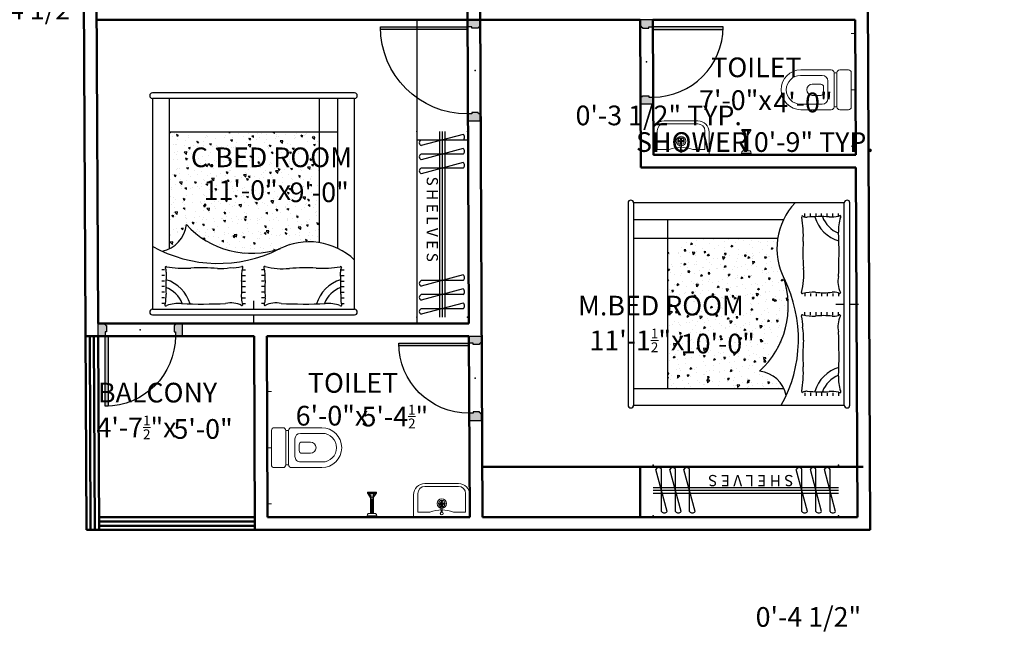
# Model space of a CAD drawing. Units: inches. Extents: x 4508 to 5907, y 877 to 1592.
# Tile 13 of 20: x 5553 to 5904, y 885 to 1107. Entities that reach past the tile are written whole.
import ezdxf

# ---------------------------------------------------------------- set-up
doc = ezdxf.new("R2010")
doc.units = ezdxf.units.IN
doc.layers.get('DEFPOINTS').update_dxf_attribs({"color": 8})
for name, color, linetype, lineweight in [('A-ANNO-DIMS', 2, 'Continuous', 18), ('A-DOOR', 4, 'Continuous', 25), ('A-FLOR-CASE', 30, 'Continuous', 25), ('A-FLOR-FIXT', 8, 'Continuous', 18), ('A-FURN', 24, 'Continuous', 18), ('A-WALL', 7, 'Continuous', 50)]:
    doc.layers.add(name, color=color, linetype=linetype, lineweight=lineweight)
doc.layers.add('doors & windows', color=30, linetype='Continuous')
doc.layers.add('furniture', color=24, linetype='Continuous')
doc.styles.get("Standard").update_dxf_attribs({"font": 'arial.ttf'})
doc.dimstyles.new('text', dxfattribs={"dimtxt": 7, "dimasz": 0, "dimexe": 3, "dimexo": 3, "dimgap": 0, "dimtad": 1, "dimtih": 1, "dimtoh": 1, "dimzin": 3, "dimdsep": 46, "dimlunit": 4, "dimtxsty": 'Standard', "dimblk": 'CLOSEDBLANK', "dimcen": 3, "dimse1": 1, "dimse2": 1, "dimsd1": 1, "dimsd2": 1, "dimclrd": 256, "dimclre": 256, "dimclrt": 256, "dimadec": 0, "dimazin": 0, "dimtfac": 0.5, "dimtofl": 0, "dimtmove": 0, "dimatfit": 3, "dimfxl": 3, "dimtolj": 1, "dimtzin": 0, "dimlwd": -1, "dimlwe": -1, "dimarcsym": 0})

# ---------------------------------------------------------------- blocks, each defined once
blk = doc.blocks.new('*D132')
at = {"layer": 'DEFPOINTS', "color": 0, "transparency": 16777216}
for p in [(5771.01, 1205.73), (5780.86, 1205.73), (5764.79, 1103.73)]:
    blk.add_point(p, dxfattribs=at)
at = {"layer": 'A-ANNO-DIMS', "color": 0, "transparency": 16777216, "insert": (5780.86, 1143.5), "char_height": 7, "attachment_point": 5}
blk.add_mtext('\\A1;8\'-6"', dxfattribs=at)
blk = doc.blocks.new('_ClosedBlank')
at = {"color": 0, "lineweight": -2}
for p, q in [((-1, 0), (0, 0)), ((0, 0), (-1, 0)), ((-1, 0), (-1, 0))]:
    blk.add_line(p, q, dxfattribs=at)
blk = doc.blocks.new('D1')
at = {"layer": 'doors & windows'}
h = blk.add_hatch(dxfattribs=at)
h.set_pattern_fill('DOTS', color=256, scale=2, angle=180, style=0)
h.set_pattern_definition([(180, (-2e-12, -4), (-0.0625, -0.125), [0, -0.125])])
h.paths.add_polyline_path([(2.5, 0), (3.5, 0), (3.5, 30.98, 0.008066), (2.5, 31)])
h = blk.add_hatch(dxfattribs=at)
h.set_pattern_fill('DOTS', color=256, scale=2, angle=180, style=0)
h.set_pattern_definition([(180, (0, -0.5), (-0.0625, -0.125), [0, -0.125])])
h.paths.add_polyline_path([(0, -4.5), (2.25, -4.5), (2.25, -4.25, 0.403966), (2.75, -3.75), (3, -3.75), (3, -1.5), (2.5, -1.5), (2.5, 0), (0, 0)])
h.paths.add_polyline_path([(36, -4.5), (36, 0), (33.5, 0), (33.5, -1.5), (33, -1.5), (33, -3.75), (33.25, -3.75, 0.403966), (33.75, -4.25), (33.75, -4.5)])
for p, q in [((0, 0), (0, -4.5)), ((36, 0), (36, -4.5))]:
    blk.add_line(p, q)
blk.add_lwpolyline([(3.5, 0), (3.5, 31), (2.5, 31), (2.5, 0)], close=True, dxfattribs=at)
for points in [[(3, -3.75), (3, -1.5), (2.5, -1.5), (2.5, 0), (0, 0)], [(33, -3.75), (33, -1.5), (33.5, -1.5), (33.5, 0), (36, 0)], [(0, -4.5), (2.25, -4.5)], [(36, -4.5), (33.75, -4.5)]]:
    blk.add_lwpolyline(points, dxfattribs=at)
for points in [[(2.25, -4.5), (2.25, -4.25, 0.403966), (2.75, -3.75), (3, -3.75)], [(33.75, -4.5), (33.75, -4.25, -0.403966), (33.25, -3.75), (33, -3.75)]]:
    blk.add_lwpolyline(points, format="xyb", dxfattribs=at)
at = {"layer": 'doors & windows', "ltscale": 6}
blk.add_arc((2.5, 0), 31, 0, 90, dxfattribs=at)
at = {"layer": 'doors & windows'}
blk.add_point((18, -2.75), dxfattribs=at)
blk = doc.blocks.new('*D134')
at = {"layer": 'DEFPOINTS', "color": 0, "transparency": 16777216}
for p in [(5644.27, 1107.42), (5631.15, 999.42), (5659.85, 999.42)]:
    blk.add_point(p, dxfattribs=at)
at = {"layer": 'A-ANNO-DIMS', "color": 0, "transparency": 16777216, "insert": (5659.85, 1046.04), "char_height": 7, "attachment_point": 5}
blk.add_mtext('\\A1;9\'-0"', dxfattribs=at)
blk = doc.blocks.new('*D135')
at = {"layer": 'DEFPOINTS', "color": 0, "transparency": 16777216}
for p in [(5712.65, 1064.65), (5580.65, 1050.69), (5712.65, 1043.18)]:
    blk.add_point(p, dxfattribs=at)
at = {"layer": 'A-ANNO-DIMS', "color": 0, "transparency": 16777216, "insert": (5634.27, 1052.65), "char_height": 7, "attachment_point": 5}
blk.add_mtext('\\A1;        C.BED ROOM\\P11\'-0"x', dxfattribs=at)
blk = doc.blocks.new('bed')
at = {"layer": 'furniture'}
h = blk.add_hatch(dxfattribs=at)
h.set_pattern_fill('AR-CONC', color=256, angle=-90, style=0)
h.set_pattern_definition([(320, (0, 2.38), (-0.6275, -7.1726), [0.75, -8.25]), (265, (0, 2.38), (7.5219, 1.3875), [0.6, -6.6]), (10.451, (-0.052, 1.782), (6.8944, -5.7851), [0.6374, -7.0114]), (316.184, (2, 2.38), (-1.6552, -10.6724), [1.125, -12.375]), (6.636, (1.862, 1.491), (9.7412, -9.3466), [0.9561, -10.5171]), (261.184, (2, 2.38), (9.7412, -9.3466), [0.9, -9.9]), (291, (1.5, 1.38), (-4.0262, -5.96907), [0.75, -8.25]), (236, (1.5, 1.38), (7.2515, -2.43315), [0.6, -6.6]), (341.451, (1.1645, 0.8826), (3.2253, -8.4022), [0.6374, -7.0114]), (307.5, (0, 2.38), (3.32894, -0.1216), [0, -6.52, 0, -6.7, 0, -6.625]), (277.5, (0, 2.38), (3.94412, -2.6307), [0, -3.82, 0, -6.37, 0, -2.525]), (237.5, (0, 4.61), (-0.22555, -5.33822), [0, -2.5, 0, -7.8, 0, -10.35]), (227.5, (0, 5.61), (1.00105, -5.83186), [0, -3.25, 0, -5.18, 0, -7.35])])
h.paths.add_polyline_path([(30.01, -68), (30.01, -26.5, 0.263043), (23.9, -35.15, 0.293424), (-9.18, -26.47, -0.156683), (-23.39, -28.72), (-23.39, -68)])
for p, q in [((0, -3), (0, 0)), ((36.01, -3), (-36.01, -3)), ((-36.01, -5), (-36.01, -80)), ((36.01, -5), (-36.01, -5)), ((0, -8), (0, -5)), ((36.01, -80), (36.01, -5)), ((-31.24, -7.07), (-32.24, -7.07)), ((-31.24, -9.07), (-32.24, -9.07)), ((-3.81, -7.07), (-2.81, -7.07)), ((-3.81, -9.07), (-2.81, -9.07)), ((3.89, -7.07), (2.89, -7.07)), ((3.89, -9.07), (2.89, -9.07)), ((31.63, -7.07), (32.63, -7.07)), ((31.63, -9.07), (32.63, -9.07)), ((-31.24, -11.07), (-32.24, -11.07)), ((-31.24, -13.07), (-32.24, -13.07)), ((-3.81, -11.07), (-2.81, -11.07)), ((-3.81, -13.07), (-2.81, -13.07)), ((3.89, -11.07), (2.89, -11.07)), ((3.89, -13.07), (2.89, -13.07)), ((31.63, -11.07), (32.63, -11.07)), ((31.63, -13.07), (32.63, -13.07)), ((-31.24, -15.07), (-32.24, -15.07)), ((-31.24, -17.07), (-32.24, -17.07)), ((-3.81, -15.07), (-2.81, -15.07)), ((-3.81, -17.07), (-2.81, -17.07)), ((3.89, -15.07), (2.89, -15.07)), ((3.89, -17.07), (2.89, -17.07)), ((31.63, -15.07), (32.63, -15.07)), ((31.63, -17.07), (32.63, -17.07)), ((-31.24, -19.07), (-32.24, -19.07)), ((-3.81, -19.07), (-2.81, -19.07)), ((3.89, -19.07), (2.89, -19.07)), ((31.63, -19.07), (32.63, -19.07)), ((-36.01, -80), (36.01, -80)), ((-36.01, -82), (36.01, -82))]:
    blk.add_line(p, q, dxfattribs=at)
at = {"layer": 'furniture', "ltscale": 5}
blk.add_line((-30.01, -26.66), (-30.01, -80), dxfattribs=at)
at = {"layer": 'furniture', "ltscale": 7}
blk.add_line((30.01, -80), (30.01, -26.5), dxfattribs=at)
at = {"layer": 'furniture', "ltscale": 0.3}
for p, q in [((-23.39, -80), (-23.39, -28.72)), ((-30.01, -68), (30.01, -68))]:
    blk.add_line(p, q, dxfattribs=at)
at = {"layer": 'furniture'}
for centre, radius, start, end in [((-35.95, -4), 1, 93.3831, 266.6169), ((35.95, -4), 1, 273.3831, 86.6169), ((-31.1, -6.57), 0.382, 35.8976, 208.6272), ((-44.44, -13.85), 14.82, 27.1629, 28.6272), ((-34.45, -3.51), 12.47, 286.0319, 344.1205), ((-26.35, 6.68), 13.76, 251.1782, 273.3982), ((-18.02, -163.6), 156.72, 87.0032, 92.7497), ((-8.03, 2.03), 9.29, 258.896, 294.7184), ((-4.03, -6.67), 0.282, 335.7259, 114.303), ((3.22, -9.94), 7.68, 155.7259, 159.0146), ((4.11, -6.67), 0.282, 65.697, 204.2741), ((-3.14, -9.94), 7.68, 20.9854, 24.2741), ((8.12, 2.03), 9.29, 245.2816, 281.104), ((18.1, -163.6), 156.72, 87.2503, 92.9968), ((34.54, -3.51), 12.47, 195.8795, 253.9681), ((26.43, 6.68), 13.76, 266.6018, 288.8218), ((31.18, -6.57), 0.382, 331.3728, 144.1024), ((44.53, -13.85), 14.82, 151.3728, 152.8371), ((-46.76, -9.65), 15.72, 357.4804, 9.3956), ((54.88, -13.16), 85.99, 178.1209, 183.3613), ((-34.45, -3.51), 9.85, 289.8695, 338.9843), ((0.25, -8.8), 4.49, 159.0146, 186.273), ((-32.82, -12.44), 28.78, 354.3784, 6.273), ((-0.17, -8.8), 4.49, 353.727, 20.9854), ((32.9, -12.44), 28.78, 173.727, 185.6216), ((34.54, -3.51), 9.85, 201.0157, 250.1305), ((-54.8, -13.16), 85.99, 356.6387, 1.8791), ((46.84, -9.65), 15.72, 170.6044, 182.5196), ((-28.62, 31.03), 42.31, 266.4836, 266.6487), ((28.7, 31.03), 42.31, 273.3513, 273.5164), ((12.28, -16.11), 16.48, 177.0317, 192.8678), ((-12.19, -16.11), 16.48, 347.1322, 2.9683), ((-31.05, -19.91), 0.291, 147.6219, 311.9343), ((-33.2, -18.55), 2.25, 327.6219, 339.2246), ((-34.13, -18.41), 3.18, 342.7809, 3.755), ((-24.4, -58.01), 38.42, 93.5164, 99.6766), ((-24.52, -56.06), 36.48, 86.4836, 93.5164), ((-18.49, 70.49), 90.23, 267.5921, 273.6329), ((-10.31, -44.95), 25.52, 75.952, 95.5452), ((-3.95, -19.99), 0.265, 231.9005, 52.8902), ((4.03, -19.99), 0.265, 127.1098, 308.0995), ((7.57, -34.68), 14.87, 87.3976, 103.1191), ((11.44, -34.81), 15.32, 84.694, 102.0355), ((18.57, 70.49), 90.23, 266.3671, 272.4079), ((24.6, -56.06), 36.48, 86.4836, 93.5164), ((24.48, -58.01), 38.42, 80.3234, 86.4836), ((31.13, -19.91), 0.291, 228.0657, 32.3781), ((34.21, -18.41), 3.18, 176.245, 197.2191), ((33.28, -18.55), 2.25, 200.7754, 212.3781), ((-19.79, -5.47), 23.53, 226.4061, 297.4441), ((12.51, -69.71), 48.38, 60.9345, 116.3227), ((0.6, -56.57), 31.65, 42.5874, 108.5034), ((34.61, -36.23), 10.76, 101.1719, 174.259), ((-35.95, -81), 1, 93.3831, 266.6169), ((35.95, -81), 1, 273.3831, 86.6169)]:
    blk.add_arc(centre, radius, start, end, dxfattribs=at)
blk = doc.blocks.new('hangers')
at = {"layer": 'furniture'}
for p, q in [((1, 7.5), (5, -7.5)), ((3, 7.5), (3, -7.5)), ((6, 7.5), (10, -7.5)), ((8, 7.5), (8, -7.5)), ((11, 7.5), (15, -7.5)), ((13, 7.5), (13, -7.5)), ((51, 7.5), (55, -7.5)), ((53, 7.5), (53, -7.5)), ((56, 7.5), (60, -7.5)), ((58, 7.5), (58, -7.5)), ((61, 7.5), (65, -7.5)), ((63, 7.5), (63, -7.5)), ((66, 1), (0, 1)), ((0, 0), (66, 0)), ((0, -1), (66, -1))]:
    blk.add_line(p, q, dxfattribs=at)
for centre, radius, start, end in [((2, 6.62), 1.33, 41.2884, 138.7116), ((7, 6.62), 1.33, 41.2884, 138.7116), ((12, 6.62), 1.33, 41.2884, 138.7116), ((52, 6.62), 1.33, 41.2884, 138.7116), ((57, 6.62), 1.33, 41.2884, 138.7116), ((62, 6.62), 1.33, 41.2884, 138.7116), ((4, -7.08), 1.08, 202.5549, 337.4451), ((9, -7.08), 1.08, 202.5549, 337.4451), ((14, -7.08), 1.08, 202.5549, 337.4451), ((54, -7.08), 1.08, 202.5549, 337.4451), ((59, -7.08), 1.08, 202.5549, 337.4451), ((64, -7.08), 1.08, 202.5549, 337.4451)]:
    blk.add_arc(centre, radius, start, end, dxfattribs=at)
for p in [(0, 9), (66, 9), (0, -9), (66, -9)]:
    blk.add_point(p, dxfattribs=at)
blk.add_text('S H E L V E S', height=4, dxfattribs=at).set_placement((16, -5.52))
blk = doc.blocks.new('D2')
at = {"layer": 'doors & windows'}
h = blk.add_hatch(dxfattribs=at)
h.set_pattern_fill('DOTS', color=256, scale=2, angle=180, style=0)
h.set_pattern_definition([(180, (0, -4), (-0.0625, -0.125), [0, -0.125])])
h.paths.add_polyline_path([(2.5, 0), (3.5, 0), (3.5, 24.98, 0.010003), (2.5, 25)])
h = blk.add_hatch(dxfattribs=at)
h.set_pattern_fill('DOTS', color=256, scale=2, angle=180, style=0)
h.set_pattern_definition([(180, (0, 0), (-0.0625, -0.125), [0, -0.125])])
edge = h.paths.add_edge_path()
edge.add_line((27.5, 0), (27.5, -1.5))
edge.add_line((27.5, -1.5), (27, -1.5))
edge.add_line((27, -1.5), (27, -3.75))
edge.add_line((27, -3.75), (27.25, -3.75))
edge.add_arc((27.76, -3.74), 0.509, 181.0059, 268.9941)
edge.add_line((27.75, -4.25), (27.75, -4.5))
edge.add_line((27.75, -4.5), (30, -4.5))
edge.add_line((30, -4.5), (30, 0))
edge.add_line((30, 0), (27.5, 0))
edge = h.paths.add_edge_path()
edge.add_line((2.5, -1.5), (2.5, 0))
edge.add_line((2.5, 0), (0, 0))
edge.add_line((0, 0), (0, -4.5))
edge.add_line((0, -4.5), (2.25, -4.5))
edge.add_line((2.25, -4.5), (2.25, -4.25))
edge.add_arc((2.24, -3.74), 0.509, 271.0059, 358.9941)
edge.add_line((2.75, -3.75), (3, -3.75))
edge.add_line((3, -3.75), (3, -1.5))
edge.add_line((3, -1.5), (2.5, -1.5))
for p, q in [((0, 0), (0, -4.5)), ((30, 0), (30, -4.5))]:
    blk.add_line(p, q)
blk.add_lwpolyline([(3.5, 0), (3.5, 25), (2.5, 25), (2.5, 0)], close=True, dxfattribs=at)
for points in [[(3, -3.75), (3, -1.5), (2.5, -1.5), (2.5, 0), (0, 0)], [(27, -3.75), (27, -1.5), (27.5, -1.5), (27.5, 0), (30, 0)], [(0, -4.5), (2.25, -4.5)], [(30, -4.5), (27.75, -4.5)]]:
    blk.add_lwpolyline(points, dxfattribs=at)
for points in [[(2.25, -4.5), (2.25, -4.25, 0.403966), (2.75, -3.75), (3, -3.75)], [(27.75, -4.5), (27.75, -4.25, -0.403966), (27.25, -3.75), (27, -3.75)]]:
    blk.add_lwpolyline(points, format="xyb", dxfattribs=at)
at = {"layer": 'doors & windows', "ltscale": 6}
blk.add_arc((2.5, 0), 25, 0, 90, dxfattribs=at)
at = {"layer": 'doors & windows'}
blk.add_point((15, -2.25), dxfattribs=at)
blk = doc.blocks.new('*D136')
at = {"layer": 'DEFPOINTS', "color": 0, "transparency": 16777216}
for p in [(5862.65, 1083.42), (5778.65, 1073.73), (5862.65, 1075.19)]:
    blk.add_point(p, dxfattribs=at)
at = {"layer": 'A-ANNO-DIMS', "color": 0, "transparency": 16777216, "insert": (5808.02, 1084.66), "char_height": 7, "attachment_point": 5}
blk.add_mtext('\\A1;       TOILET\\P7\'-0"x', dxfattribs=at)
blk = doc.blocks.new('*D137')
at = {"layer": 'DEFPOINTS', "color": 0, "transparency": 16777216}
for p in [(5825.34, 1107.42), (5825.34, 1059.42), (5832.08, 1059.42)]:
    blk.add_point(p, dxfattribs=at)
at = {"layer": 'A-ANNO-DIMS', "color": 0, "transparency": 16777216, "insert": (5832.08, 1078.01), "char_height": 7, "attachment_point": 5}
blk.add_mtext('\\A1;4\'-0"', dxfattribs=at)
blk = doc.blocks.new('commode')
for p, q in [((-7.09, 19.41), (-7.09, 8.61)), ((-5.09, 11.81), (-5.09, 19.57)), ((5.09, 11.81), (5.09, 19.57)), ((7.09, 19.41), (7.09, 8.61)), ((-2, 12.37), (-2, 15.37)), ((2, 12.37), (2, 15.37)), ((-1, 11.37), (1, 11.37)), ((-6.09, 7.61), (6.09, 7.61)), ((-6.09, 6.61), (-6.09, 7.61)), ((-3.15, 9.87), (3.15, 9.87)), ((6.09, 7.61), (6.09, 6.61)), ((-7.09, 2.5), (-7.09, 5.61)), ((-6.09, 6.61), (6.09, 6.61)), ((7.09, 2.5), (7.09, 5.61)), ((-20, 1.5), (-20, 0)), ((-6.09, 1.5), (6.09, 1.5)), ((0, 1.5), (0, 0)), ((20, 1.5), (20, 0))]:
    blk.add_line(p, q)
for centre, radius, start, end in [((0, 19.41), 7.09, 0, 180), ((0, 19.57), 5.09, 0, 180), ((0, 15.37), 2, 0, 180), ((-3.15, 11.81), 1.94, 180, 270), ((-1, 12.37), 1, 180, 270), ((1, 12.37), 1, 270, 0), ((3.15, 11.81), 1.94, 270, 0), ((-6.09, 8.61), 1, 180, 270), ((6.09, 8.61), 1, 270, 0), ((-6.09, 5.61), 1, 90, 180), ((6.09, 5.61), 1, 0, 90), ((-6.09, 2.5), 1, 180, 270), ((6.09, 2.5), 1, 270, 0)]:
    blk.add_arc(centre, radius, start, end)
blk = doc.blocks.new('wash basin 1')
for p, q in [((-8.5, 8.5), (-1.85, 8.5)), ((0, 10), (-8, 10)), ((-1.85, 8.5), (-1.85, 4.19)), ((0, 10), (0, -10)), ((-12, 6), (-12, -6)), ((-11, 6), (-11, -6)), ((-1.85, -8.5), (-1.85, -4.19)), ((-8.5, -8.5), (-1.85, -8.5)), ((0, -10), (-8, -10))]:
    blk.add_line(p, q)
blk.add_lwpolyline([(-1.83, 0.11), (-5.25, 0.25), (-5.23, -0.38), (-1.8, -0.19)])
for centre, radius in [((-4.87, 0), 1.68), ((-4.87, 0), 1.18), ((-5.63, 0), 0.25), ((-4.87, 0.75), 0.25), ((-4.87, 0), 0.25), ((-4.19, 0), 0.25), ((-1.34, 0), 0.5), ((-4.87, -0.72), 0.25)]:
    blk.add_circle(centre, radius)
for centre, radius, start, end in [((-8, 6), 4, 90, 180), ((-8.5, 6), 2.5, 90, 180), ((8.89, 0), 11.53, 158.7059, 201.2941), ((-8, -6), 4, 180, 270), ((-8.5, -6), 2.5, 180, 270)]:
    blk.add_arc(centre, radius, start, end)
blk = doc.blocks.new('tap & shower')
for p, q in [((1.71, 0), (-1.71, 0)), ((-1.71, 0), (-1.71, -0.5)), ((1.71, 0), (1.71, -0.5)), ((1.71, -0.5), (-1.71, -0.5)), ((1.31, -1.4), (-1.31, -1.4)), ((-0.5, -6.44), (-0.5, -1.4)), ((-0.42, -6.44), (-0.42, -1.4)), ((-0.32, -0.5), (0.32, -0.5)), ((-0.3, -6.44), (-0.3, -1.4)), ((-0.14, -6.44), (-0.14, -1.4)), ((0.14, -6.44), (0.14, -1.4)), ((0.3, -6.44), (0.3, -1.4)), ((0.42, -6.44), (0.42, -1.4)), ((0.5, -6.44), (0.5, -1.4)), ((-1.48, -8.46), (-0.47, -6.98)), ((-0.41, -6.98), (-0.94, -8.46)), ((-0.56, -6.44), (0.56, -6.44)), ((-0.56, -6.98), (-0.56, -6.44)), ((-0.56, -6.98), (0.56, -6.98)), ((-0.29, -6.98), (-0.4, -8.46)), ((0.29, -6.98), (0.4, -8.46)), ((0.41, -6.98), (0.94, -8.46)), ((1.48, -8.46), (0.47, -6.98)), ((0.56, -6.98), (0.56, -6.44)), ((-1.62, -8.87), (-1.62, -8.6)), ((-1.48, -8.46), (1.48, -8.46)), ((-1.48, -9), (-1.48, -8.46)), ((-1.48, -9), (1.48, -9)), ((-1.43, -9), (-1.43, -8.46)), ((-1.37, -9), (-1.37, -8.46)), ((-1.32, -9), (-1.32, -8.46)), ((-1.27, -9), (-1.27, -8.46)), ((-1.21, -9), (-1.21, -8.46)), ((-1.16, -9), (-1.16, -8.46)), ((-1.1, -9), (-1.1, -8.46)), ((-1.05, -9), (-1.05, -8.46)), ((-1, -9), (-1, -8.46)), ((-0.94, -9), (-0.94, -8.46)), ((-0.89, -9), (-0.89, -8.46)), ((-0.84, -9), (-0.84, -8.46)), ((-0.78, -9), (-0.78, -8.46)), ((-0.73, -9), (-0.73, -8.46)), ((-0.67, -9), (-0.67, -8.46)), ((-0.62, -9), (-0.62, -8.46)), ((-0.57, -9), (-0.57, -8.46)), ((-0.51, -9), (-0.51, -8.46)), ((-0.46, -9), (-0.46, -8.46)), ((-0.4, -9), (-0.4, -8.46)), ((-0.35, -9), (-0.35, -8.46)), ((-0.3, -9), (-0.3, -8.46)), ((-0.24, -9), (-0.24, -8.46)), ((-0.19, -9), (-0.19, -8.46)), ((-0.13, -9), (-0.13, -8.46)), ((-0.08, -9), (-0.08, -8.46)), ((-0.03, -9), (-0.03, -8.46)), ((0.03, -9), (0.03, -8.46)), ((0.08, -9), (0.08, -8.46)), ((0.13, -9), (0.13, -8.46)), ((0.19, -9), (0.19, -8.46)), ((0.24, -9), (0.24, -8.46)), ((0.3, -9), (0.3, -8.46)), ((0.35, -9), (0.35, -8.46)), ((0.4, -9), (0.4, -8.46)), ((0.46, -9), (0.46, -8.46)), ((0.51, -9), (0.51, -8.46)), ((0.57, -9), (0.57, -8.46)), ((0.62, -9), (0.62, -8.46)), ((0.67, -9), (0.67, -8.46)), ((0.73, -9), (0.73, -8.46)), ((0.78, -9), (0.78, -8.46)), ((0.84, -9), (0.84, -8.46)), ((0.89, -9), (0.89, -8.46)), ((0.94, -9), (0.94, -8.46)), ((1, -9), (1, -8.46)), ((1.05, -9), (1.05, -8.46)), ((1.1, -9), (1.1, -8.46)), ((1.16, -9), (1.16, -8.46)), ((1.21, -9), (1.21, -8.46)), ((1.27, -9), (1.27, -8.46)), ((1.32, -9), (1.32, -8.46)), ((1.37, -9), (1.37, -8.46)), ((1.43, -9), (1.43, -8.46)), ((1.48, -9), (1.48, -8.46)), ((1.62, -8.87), (1.62, -8.6))]:
    blk.add_line(p, q)
for centre, radius, start, end in [((-0.02, -0.29), 1.7, 187.1825, 220.9028), ((0.02, -0.29), 1.7, 319.0972, 352.8175), ((-1.48, -8.6), 0.135, 90, 180), ((-1.48, -8.87), 0.135, 180, 270), ((1.48, -8.6), 0.135, 0, 90), ((1.48, -8.87), 0.135, 270, 0)]:
    blk.add_arc(centre, radius, start, end)
blk = doc.blocks.new('*D140')
at = {"layer": 'DEFPOINTS', "color": 0, "transparency": 16777216}
for p in [(5713.36, 962.94), (5713.36, 954.9), (5641.38, 948.51)]:
    blk.add_point(p, dxfattribs=at)
at = {"layer": 'A-ANNO-DIMS', "color": 0, "transparency": 16777216, "insert": (5664.41, 972.41), "char_height": 7, "attachment_point": 5}
blk.add_mtext('\\A1;       TOILET\\P6\'-0"x', dxfattribs=at)
blk = doc.blocks.new('*D141')
at = {"layer": 'DEFPOINTS', "color": 0, "transparency": 16777216}
for p in [(5670.26, 994.92), (5672.15, 930.42), (5686.79, 930.42)]:
    blk.add_point(p, dxfattribs=at)
at = {"layer": 'A-ANNO-DIMS', "color": 0, "transparency": 16777216, "insert": (5686.79, 966.25), "char_height": 7, "attachment_point": 5}
blk.add_mtext('\\A1;5\'-4{\\H0.5x;\\S1/2;}"', dxfattribs=at)
blk = doc.blocks.new('*D138')
at = {"layer": 'DEFPOINTS', "color": 0, "transparency": 16777216}
for p in [(5632.76, 959.84), (5632.76, 958.24), (5577.26, 956.6)]:
    blk.add_point(p, dxfattribs=at)
at = {"layer": 'A-ANNO-DIMS', "color": 0, "transparency": 16777216, "insert": (5594.82, 968.24), "char_height": 7, "attachment_point": 5}
blk.add_mtext('\\A1;       BALCONY\\P4\'-7{\\H0.5x;\\S1/2;}"x', dxfattribs=at)
blk = doc.blocks.new('*D139')
at = {"layer": 'DEFPOINTS', "color": 0, "transparency": 16777216}
for p in [(5600.67, 994.92), (5600.67, 934.92), (5618.52, 934.92)]:
    blk.add_point(p, dxfattribs=at)
at = {"layer": 'A-ANNO-DIMS', "color": 0, "transparency": 16777216, "insert": (5618.52, 961.85), "char_height": 7, "attachment_point": 5}
blk.add_mtext('\\A1;5\'-0"', dxfattribs=at)
blk = doc.blocks.new('*D142')
at = {"layer": 'DEFPOINTS', "color": 0, "transparency": 16777216}
for p in [(5790.24, 1046.47), (5785.03, 926.47), (5801.77, 926.47)]:
    blk.add_point(p, dxfattribs=at)
at = {"layer": 'A-ANNO-DIMS', "color": 0, "transparency": 16777216, "insert": (5801.77, 992.23), "char_height": 7, "attachment_point": 5}
blk.add_mtext('\\A1;10\'-0"', dxfattribs=at)
blk = doc.blocks.new('*D143')
at = {"layer": 'DEFPOINTS', "color": 0, "transparency": 16777216}
for p in [(5851.78, 989.21), (5718.28, 986.04), (5851.78, 974.04)]:
    blk.add_point(p, dxfattribs=at)
at = {"layer": 'A-ANNO-DIMS', "color": 0, "transparency": 16777216, "insert": (5772.96, 999.2), "char_height": 7, "attachment_point": 5}
blk.add_mtext('\\A1;        M.BED ROOM\\P11\'-1{\\H0.5x;\\S1/2;}"x', dxfattribs=at)
blk = doc.blocks.new('*D160')
at = {"layer": 'DEFPOINTS', "color": 0, "transparency": 16777216}
for p in [(5813.62, 1068.42), (5813.62, 1059.42), (5814.97, 1059.42)]:
    blk.add_point(p, dxfattribs=at)
at = {"layer": 'A-ANNO-DIMS', "transparency": 16777216, "insert": (5814.97, 1063.92), "char_height": 7, "attachment_point": 5}
blk.add_mtext('\\A1;SHOWER 0\'-9" TYP.', dxfattribs=at)
blk = doc.blocks.new('*D161')
at = {"layer": 'DEFPOINTS', "color": 0, "transparency": 16777216}
for p in [(5813.62, 1069.77), (5810.21, 1068.42), (5813.62, 1068.42)]:
    blk.add_point(p, dxfattribs=at)
at = {"layer": 'A-ANNO-DIMS', "transparency": 16777216, "insert": (5780.72, 1073.39), "char_height": 7, "attachment_point": 5}
blk.add_mtext('\\A1;0\'-3 1/2" TYP.', dxfattribs=at)
blk = doc.blocks.new('*D192')
at = {"layer": 'DEFPOINTS', "color": 0, "transparency": 16777216}
for p in [(5851.47, 930.42), (5855.99, 925.92), (5855.99, 891.35)]:
    blk.add_point(p, dxfattribs=at)
at = {"layer": 'A-ANNO-DIMS', "transparency": 16777216, "insert": (5834.01, 894.97), "char_height": 7, "attachment_point": 5}
blk.add_mtext('\\A1;0\'-4 1/2"', dxfattribs=at)
blk = doc.blocks.new('*D193')
at = {"layer": 'DEFPOINTS', "color": 0, "transparency": 16777216}
for p in [(5539.44, 1111.92), (5580.63, 1111.92), (5580.65, 1107.42)]:
    blk.add_point(p, dxfattribs=at)
at = {"layer": 'A-ANNO-DIMS', "transparency": 16777216, "insert": (5556.9, 1111.04), "char_height": 7, "attachment_point": 5}
blk.add_mtext('\\A1;0\'-4 1/2"', dxfattribs=at)
blk = doc.blocks.new('*D194')
at = {"layer": 'DEFPOINTS', "color": 0, "transparency": 16777216}
for p in [(5854.266243, 1573.916611), (5890.541519, 1573.916611), (5855.991519, 925.916611)]:
    blk.add_point(p, dxfattribs=at)
at = {"layer": 'A-ANNO-DIMS', "transparency": 16777216, "insert": (5890.541519, 1249.916611), "char_height": 7, "attachment_point": 5}
blk.add_mtext('\\A1;54\'-0"', dxfattribs=at)

msp = doc.modelspace()

# ---------------------------------------------------------------- linework, layer by layer
at = {"layer": 'A-FLOR-CASE'}
for p, q in [((5694.65, 1107.417), (5694.65, 999.417)), ((5712.65, 1064.646), (5694.65, 1064.646))]:
    msp.add_line(p, q, dxfattribs=at)
at = {"layer": 'A-WALL'}
for p, q in [((5576.989, 925.917), (5573.989, 1573.917)), ((5855.992, 925.917), (5854.266, 1298.576)), ((5581.148, 999.417), (5579.787, 1293.417)), ((5713.15, 999.417), (5712.629, 1111.917)), ((5717.969, 930.417), (5717.129, 1111.917)), ((5580.648, 1107.417), (5774.15, 1107.417)), ((5774.393, 1054.917), (5774.15, 1107.417)), ((5778.873, 1059.417), (5778.65, 1107.417)), ((5778.65, 1107.417), (5850.651, 1107.417)), ((5850.873, 1059.417), (5850.651, 1107.417)), ((5778.873, 1059.417), (5850.873, 1059.417)), ((5774.393, 1054.917), (5850.894, 1054.917)), ((5851.471, 930.417), (5850.894, 1054.917)), ((5581.148, 999.417), (5713.15, 999.417)), ((5576.669, 994.917), (5636.67, 994.917)), ((5578.489, 925.903), (5578.169, 994.903)), ((5579.989, 925.91), (5579.669, 994.91)), ((5581.489, 925.917), (5581.169, 994.917)), ((5636.989, 925.917), (5636.67, 994.917)), ((5641.468, 930.417), (5641.17, 994.917)), ((5641.17, 994.917), (5713.171, 994.917)), ((5713.469, 930.417), (5713.171, 994.917)), ((5717.886, 948.417), (5853.485, 948.417)), ((5774.119, 948.417), (5774.119, 930.417)), ((5636.968, 930.417), (5581.468, 930.417)), ((5636.975, 928.917), (5581.468, 928.917)), ((5713.469, 930.417), (5641.468, 930.417)), ((5851.471, 930.417), (5717.969, 930.417)), ((5855.992, 925.917), (5576.989, 925.917)), ((5636.982, 927.417), (5581.468, 927.417))]:
    msp.add_line(p, q, dxfattribs=at)

# ---------------------------------------------------------------- block references
at = {"layer": 'A-DOOR', "xscale": -1}
for name, p, rotation in [('D1', (5712.65, 1107.417), 90), ('D2', (5581.169, 994.917), 180), ('D2', (5713.171, 994.917), 90)]:
    msp.add_blockref(name, p, dxfattribs=dict(at, rotation=rotation))
at = {"layer": 'A-DOOR', "rotation": 270}
msp.add_blockref('D2', (5778.65, 1107.417), dxfattribs=at)
at = {"layer": 'A-FLOR-FIXT'}
for name, p, rotation in [('commode', (5850.767, 1082.508), 90), ('wash basin 1', (5788.65, 1059.417), 270), ('commode', (5641.354, 955.193), 270), ('wash basin 1', (5703.469, 930.417), 270)]:
    msp.add_blockref(name, p, dxfattribs=dict(at, rotation=rotation))
at = {"layer": 'A-FLOR-FIXT', "xscale": -1, "rotation": 180}
for p in [(5811.913, 1059.417), (5678.625, 930.417)]:
    msp.add_blockref('tap & shower', p, dxfattribs=at)
at = {"layer": 'A-FURN'}
for name, p, rotation in [('bed', (5636.461, 999.417), 180), ('hangers', (5703.65, 1067.646), 270), ('bed', (5851.784, 1006.282), 270), ('hangers', (5844.702, 939.958), 180)]:
    msp.add_blockref(name, p, dxfattribs=dict(at, rotation=rotation))

# ---------------------------------------------------------------- dimensions: what is measured, and where the dimension line sits
at = {"layer": 'A-ANNO-DIMS'}
for base, p1, p2, picture, middle in [((5890.542, 1573.917), (5855.992, 925.917), (5854.266, 1573.917), '*D194', (5890.542, 1249.917)), ((5539.439, 1111.917), (5580.648, 1107.417), (5580.627, 1111.917), '*D193', (5556.898, 1111.036))]:
    dim = msp.add_linear_dim(base=base, p1=p1, p2=p2, angle=90, dimstyle='text', override={"dimdec": 1, "dimlfac": 1, "dimrnd": 0, "dimzin": 1, "dimdsep": 46, "dimlunit": 4, "dimfrac": 2}, dxfattribs=at)
    dim.commit()
    dim.dimension.update_dxf_attribs({"geometry": picture, "text_midpoint": middle})
for base, p1, p2, picture, middle in [((5780.857, 1205.735), (5764.789, 1103.735), (5771.013, 1205.735), '*D132', (5780.857, 1143.502)), ((5659.853, 999.417), (5644.265, 1107.417), (5631.15, 999.417), '*D134', (5659.853, 1046.04)), ((5832.084, 1059.417), (5825.336, 1107.417), (5825.336, 1059.417), '*D137', (5832.084, 1078.014)), ((5801.771, 926.471), (5790.24, 1046.471), (5785.034, 926.471), '*D142', (5801.771, 992.231)), ((5618.519, 934.917), (5600.67, 994.917), (5600.67, 934.917), '*D139', (5618.519, 961.854)), ((5686.792, 930.417), (5670.265, 994.917), (5672.151, 930.417), '*D141', (5686.792, 966.246))]:
    dim = msp.add_linear_dim(base=base, p1=p1, p2=p2, angle=90, dimstyle='text', override={"dimclrd": 0, "dimclre": 0, "dimclrt": 0}, dxfattribs=at)
    dim.commit()
    dim.dimension.update_dxf_attribs({"geometry": picture, "text_midpoint": middle, "dimtype": 160})
for base, p1, p2, text, picture, middle in [((5862.65, 1075.192), (5778.65, 1073.732), (5862.65, 1083.417), '       TOILET\\P<>x', '*D136', (5808.02, 1075.192)), ((5712.65, 1043.18), (5580.65, 1050.69), (5712.65, 1064.646), '        C.BED ROOM\\P<>x', '*D135', (5634.269, 1043.18)), ((5851.784, 989.21), (5718.284, 986.042), (5851.784, 974.042), '        M.BED ROOM\\P<>x', '*D143', (5772.962, 989.21)), ((5713.356, 962.941), (5641.385, 948.506), (5713.356, 954.899), '       TOILET\\P<>x', '*D140', (5664.413, 962.941)), ((5632.765, 958.242), (5577.265, 956.604), (5632.765, 959.845), '       BALCONY\\P<>x', '*D138', (5594.818, 958.242))]:
    dim = msp.add_linear_dim(base=base, p1=p1, p2=p2, text=text, dimstyle='text', override={"dimclrd": 0, "dimclre": 0, "dimclrt": 0}, dxfattribs=at)
    dim.commit()
    dim.dimension.update_dxf_attribs({"geometry": picture, "text_midpoint": middle, "dimtype": 160})
dim = msp.add_linear_dim(base=(5813.621, 1069.767), p1=(5810.205, 1068.417), p2=(5813.621, 1068.417), text='<> TYP.', dimstyle='text', override={"dimdec": 1, "dimrnd": 0, "dimzin": 1, "dimlunit": 4, "dimfrac": 2}, dxfattribs=at)
dim.commit()
dim.dimension.update_dxf_attribs({"geometry": '*D161', "text_midpoint": (5780.715, 1073.388)})
dim = msp.add_linear_dim(base=(5814.971, 1059.417), p1=(5813.621, 1068.417), p2=(5813.621, 1059.417), angle=270, text='SHOWER <> TYP.', dimstyle='text', override={"dimdec": 1, "dimrnd": 0, "dimzin": 1, "dimlunit": 4, "dimfrac": 2}, dxfattribs=at)
dim.commit()
dim.dimension.update_dxf_attribs({"geometry": '*D160', "text_midpoint": (5814.971, 1063.917)})
dim = msp.add_linear_dim(base=(5855.992, 891.353), p1=(5851.471, 930.417), p2=(5855.992, 925.917), dimstyle='text', override={"dimdec": 1, "dimlfac": 1, "dimrnd": 0, "dimzin": 1, "dimdsep": 46, "dimlunit": 4, "dimfrac": 2}, dxfattribs=at)
dim.commit()
dim.dimension.update_dxf_attribs({"geometry": '*D192', "text_midpoint": (5834.011, 894.972)})

doc.saveas('drawing.dxf')
